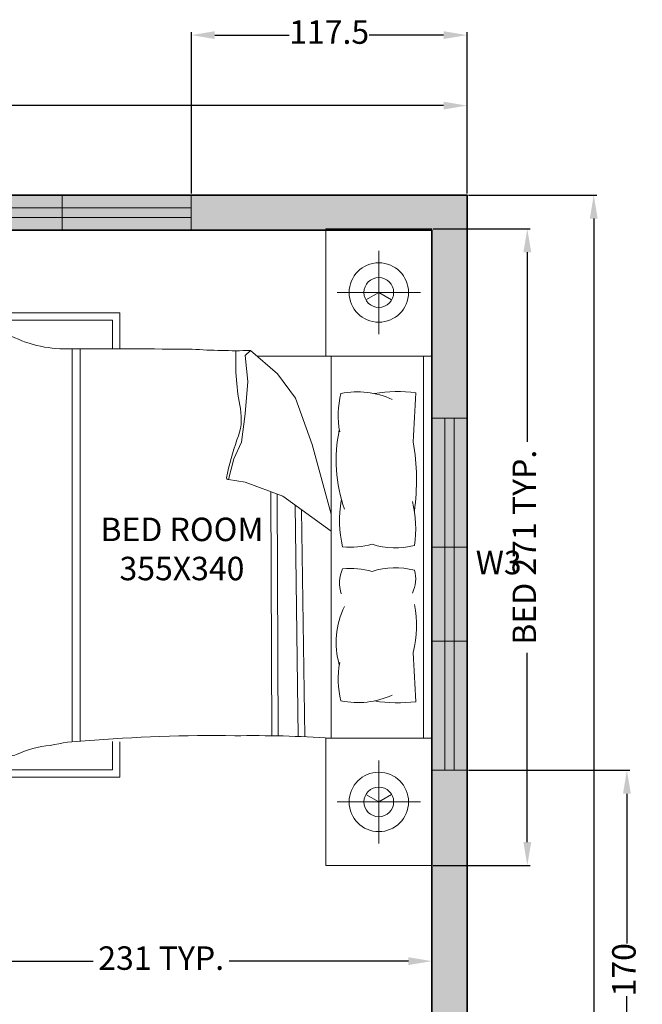
# Model space of a CAD drawing. Units: centimetres. Extents: x 2401 to 3632, y 2122 to 3526.
# Tile 10 of 10: x 3055 to 3320, y 3106 to 3526. Entities that reach past the tile are written whole.
import ezdxf

# ---------------------------------------------------------------- set-up
doc = ezdxf.new("R2010")
doc.units = ezdxf.units.CM
for name, color, linetype, lineweight in [('A-ANNO-DIMS', 9, 'Continuous', 18), ('A-ANNO-TEXT', 9, 'Continuous', 18), ('A-AREA-IDEN', 9, 'Continuous', 25), ('A-FURN', 9, 'Continuous', 18), ('A-GLAZ', 4, 'Continuous', 18), ('A-WALL', 7, 'Continuous', 35)]:
    doc.layers.add(name, color=color, linetype=linetype, lineweight=lineweight)
doc.layers.add('A-GLAZ-PATT', color=251, linetype='Continuous', lineweight=13, true_color=0x636466)
doc.layers.add('A-WALL-PATT', color=18, linetype='Continuous', lineweight=13, true_color=0x000000)
doc.styles.get("Standard").update_dxf_attribs({"font": 'arial.ttf'})
doc.dimstyles.new('ISO-25', dxfattribs={"dimtxt": 10, "dimasz": 10, "dimexe": 1.25, "dimexo": 0.625, "dimtad": 0, "dimtxsty": 'Standard', "dimcen": 2.5, "dimadec": 0, "dimazin": 0, "dimtfac": 1, "dimtmove": 0, "dimatfit": 3, "dimfxl": 1, "dimarcsym": 0})

# ---------------------------------------------------------------- blocks, each defined once
blk = doc.blocks.new('bed')
for p, q in [((3025.77, 3949.95), (3025.77, 3649.95)), ((3000.77, 3900.35), (3000.77, 3939.55)), ((2981.17, 3919.95), (3020.37, 3919.95)), ((2770.64, 3910.36), (2878.71, 3910.36)), ((2770.64, 3691.65), (2770.64, 3910.36)), ((2878.71, 3910.36), (2878.71, 3893.39)), ((2774.11, 3906.88), (2774.11, 3695.12)), ((2875.23, 3906.88), (2774.11, 3906.88)), ((2875.23, 3893.39), (2875.23, 3906.88)), ((2856.25, 3708.31), (2856.25, 3893.41)), ((2860, 3708.59), (2860, 3893.41)), ((2937.86, 3890.21), (2940.29, 3892.64)), ((2940.29, 3892.64), (2953.05, 3881.7)), ((2939.08, 3878.06), (2937.86, 3890.21)), ((3025.77, 3889.95), (2943.43, 3889.95)), ((2978.36, 3889.95), (2978.36, 3709.95)), ((3021.92, 3709.95), (3021.92, 3889.95)), ((2804.53, 3877.32), (2807.92, 3877.98)), ((2937.86, 3862.87), (2939.08, 3878.06)), ((2953.05, 3881.7), (2961.55, 3870.16)), ((2961.55, 3870.16), (2969.44, 3848.28)), ((2826.78, 3739.05), (2826.78, 3860.86)), ((2936.04, 3849.5), (2937.86, 3862.87)), ((2804.53, 3856.35), (2807.92, 3855.69)), ((2932.4, 3841.6), (2936.04, 3849.5)), ((2969.44, 3848.28), (2978.36, 3815.57)), ((2929.97, 3831.88), (2932.4, 3841.6)), ((2937.86, 3830.66), (2929.97, 3831.88)), ((2955.47, 3823.98), (2937.86, 3830.66)), ((2950.29, 3711.02), (2949.82, 3826.13)), ((2953.37, 3711.03), (2952.92, 3824.95)), ((2978.36, 3807.54), (2955.47, 3823.98)), ((2962.82, 3710.88), (2961.28, 3819.81)), ((2965.89, 3710.76), (2964.4, 3817.57)), ((2804.53, 3745.65), (2807.92, 3746.31)), ((2804.53, 3724.68), (2807.92, 3724.02)), ((2875.23, 3695.12), (2875.23, 3708.35)), ((2878.71, 3708.28), (2878.71, 3691.65)), ((3000.77, 3699.55), (3000.77, 3660.35)), ((2774.11, 3695.12), (2875.23, 3695.12)), ((2878.71, 3691.65), (2770.64, 3691.65)), ((2981.17, 3679.95), (3020.37, 3679.95))]:
    blk.add_line(p, q)
for points in [[(2975.77, 3889.95), (2975.77, 3949.95), (3025.77, 3949.95)], [(3000.77, 3919.95), (2994.7, 3916.45)], [(3000.77, 3919.95), (3006.83, 3916.45)], [(3025.77, 3709.95), (2975.77, 3709.95), (2975.77, 3649.95), (3025.77, 3649.95)], [(3000.77, 3679.95), (2994.7, 3683.45)], [(3000.77, 3679.95), (3006.83, 3683.45)]]:
    blk.add_lwpolyline(points)
for points in [[(2912.82, 3893.27, 0.001242), (2855.9, 3893.41, -0.127202), (2827.53, 3899.43)], [(3018.29, 3872.72, 0.074897), (2998.69, 3872.36, -0.472817)], [(2997.6, 3801.36, 0.14099), (3017.59, 3800.76, 0.235245)], [(2997.6, 3788.55, -0.14099), (3017.59, 3789.15, -0.235245)], [(3018.29, 3727.19, -0.074897), (2998.69, 3727.55, 0.472817)], [(2862.36, 3708.67, 0.056112), (2845.85, 3706.5, 0.095341), (2829.95, 3702.28)]]:
    blk.add_lwpolyline(points, format="xyb")
for centre, radius in [((3000.77, 3919.95), 14), ((3000.77, 3919.95), 7), ((2785.6, 3864.98), 0.764), ((2793.66, 3859.99), 0.764), ((2793.66, 3742.02), 0.764), ((2785.6, 3737.02), 0.764), ((3000.77, 3679.95), 14), ((3000.77, 3679.95), 7)]:
    blk.add_circle(centre, radius)
for centre, radius, start, end in [((2760.03, 3923.26), 23.79, 306.3036, 316.4814), ((2763.59, 3916.39), 19.09, 303.4617, 330.1116), ((2768.83, 3936.05), 39.18, 277.745, 311.8856), ((2764.96, 3869.02), 39.18, 34.3865, 68.5908), ((2827.73, 3896.66), 2.77, 93.98, 207.3412), ((2768, 3905.7), 15.93, 292.5547, 318.9546), ((2776.56, 3949.33), 54.2, 267.4081, 273.6519), ((2514.5, 3864.44), 312.3, 359.3433, 5.6887), ((2932.84, 4167.71), 275.17, 265.8294, 271.553), ((3046.53, 3887.51), 113.22, 177.4519, 191.3392), ((2796.37, 3886.9), 4.34, 77.7115, 159.0387), ((2794.02, 3891.25), 3.27, 238.4633, 358.2869), ((2804.75, 3884.63), 9.91, 138.8402, 177.9352), ((2798.78, 3888.31), 3.2, 117.6827, 223.7762), ((2798.06, 3887.99), 3.25, 2.9516, 103.728), ((2824.04, 3897.09), 27.41, 192.5173, 207.1824), ((2793.67, 3886.12), 6.19, 345.4653, 54.2343), ((2803, 3894.63), 6.69, 211.3827, 255.2969), ((2804.28, 3884.18), 4.5, 350.264, 160.8688), ((2799.41, 3885.11), 2.76, 333.9755, 53.2681), ((2815.84, 3882.53), 7.17, 84.9449, 172.8857), ((2816.56, 3884.61), 5.07, 354.4856, 91.0538), ((2805.66, 3897.83), 22.71, 303.6671, 333.2997), ((2795.33, 3884.97), 0.487, 177.9352, 11.4834), ((2795.58, 3885.02), 0.236, 11.4834, 127.9409), ((2796.77, 3886.39), 0.424, 223.7762, 159.7183), ((2805.64, 3885.26), 5.62, 175.969, 254.3045), ((2798.17, 3879.2), 5.99, 6.1662, 51.5825), ((2814.2, 3893.11), 14.16, 211.2614, 251.7045), ((2817.43, 3883.78), 8.71, 182.3591, 234.0401), ((2818.55, 3879.71), 6.96, 111.5819, 201.4221), ((2812.81, 3886.16), 9.02, 265.2933, 346.921), ((2813.05, 3893.24), 16.1, 236.2883, 266.5076), ((2810.99, 3881.04), 7.46, 209.9085, 343.1337), ((2824.57, 3889.51), 12.43, 238.8218, 279.1554), ((2819.17, 3867.4), 11.57, 55.785, 94.7304), ((2775.06, 3890.75), 28.48, 313.1541, 322.0459), ((2796.01, 3873.64), 0.586, 142.4737, 265.053), ((2796.78, 3873.76), 1.26, 127.7621, 169.0403), ((2796.11, 3874.82), 1.78, 265.053, 338.3618), ((2798.46, 3872.39), 2.32, 113.4276, 137.6104), ((2798.2, 3874.8), 0.764, 183.2768, 356.7232), ((2798.76, 3873.41), 1.25, 139.7889, 227.6792), ((2795.81, 3873.43), 2.5, 353.0852, 15.7171), ((2797.45, 3873.13), 1.58, 350.3487, 43.6538), ((2800.38, 3874.76), 1.84, 198.7263, 262.5032), ((2798.92, 3873.91), 0.73, 1.1081, 91.8675), ((2800.29, 3873.51), 0.59, 255.2356, 54.9248), ((2799.38, 3873.74), 1.27, 11.5637, 52.6358), ((2814.13, 3876.31), 1.86, 167.3041, 285.1471), ((2819.17, 3867.4), 11.57, 122.7011, 126.3445), ((2821.34, 3879.88), 9.56, 199.2822, 299.1751), ((2816.22, 3868.58), 6.15, 41.5653, 105.1471), ((2819.61, 3881.32), 8.62, 277.436, 299.9149), ((2823.47, 3874.11), 3.61, 30.0293, 52.325), ((2786.72, 3869.91), 0.853, 124.3538, 214.3923), ((2787.97, 3869.78), 1.99, 190.3057, 287.1958), ((2788.54, 3870.49), 2.31, 176.9701, 248.2913), ((2805.02, 3882.67), 22.32, 212.6784, 216.3746), ((2787.76, 3869.95), 0.883, 216.3746, 291.7548), ((2789.87, 3869.34), 1.99, 122.8155, 187.3992), ((2788.34, 3868.51), 0.666, 289.3605, 111.7548), ((2788.84, 3868.51), 0.666, 221.8703, 44.2646), ((2790.75, 3869.08), 2.31, 109.4799, 177.6828), ((2789.51, 3870.54), 0.853, 56.8636, 146.9021), ((2789.95, 3869.59), 0.883, 148.8844, 224.2646), ((2808.3, 3858.51), 22.32, 145.1882, 148.8844), ((2795.58, 3857.56), 12.46, 94.756, 119.2041), ((2822.1, 3839.62), 40.99, 132.2412, 142.1744), ((2801.41, 3872.25), 8.46, 178.3264, 187.1302), ((2792.27, 3871.07), 1.58, 11.3256, 64.4621), ((2797.62, 3873.34), 4.74, 190.2588, 210.656), ((2794.44, 3871.41), 1.44, 188.3432, 274.2869), ((2795.7, 3872.2), 2.51, 210.656, 242.6341), ((2797.6, 3874.36), 4.82, 218.2101, 226.3071), ((2794.04, 3870.31), 0.611, 325.7657, 67.4417), ((2796.2, 3845.18), 24.85, 73.5842, 93.8277), ((2798.36, 3872.98), 0.658, 227.6792, 350.3487), ((2811.5, 3870.46), 8.46, 178.3264, 187.1302), ((2802.37, 3869.29), 1.58, 11.3256, 64.4621), ((2807.71, 3871.55), 4.74, 190.2588, 210.656), ((2804.53, 3869.62), 1.44, 188.3432, 274.2869), ((2805.8, 3870.42), 2.51, 210.656, 242.6341), ((2807.7, 3872.58), 4.82, 218.2101, 226.3071), ((2804.13, 3868.53), 0.611, 325.7657, 67.4417), ((2824.18, 3875.64), 4.49, 221.5653, 293.8354), ((2823.47, 3874.11), 3.61, 314.4517, 333.558), ((3021.8, 3862.02), 40.2, 165.1039, 191.0369), ((2990.83, 3834.5), 38.67, 65.1316, 101.7583), ((5873.3, 3707.37), 2859.79, 176.68521, 177.14978), ((2783.42, 3863.83), 0.586, 142.4737, 265.053), ((2784.19, 3863.94), 1.26, 61.2196, 169.0403), ((2783.52, 3865.01), 1.78, 265.053, 338.3618), ((2785.02, 3866.54), 1.51, 157.4086, 261.4386), ((2784.17, 3866.59), 0.757, 58.0499, 135.6268), ((2785.87, 3862.58), 2.32, 113.4276, 137.6104), ((2784.96, 3866.11), 0.506, 172.906, 277.132), ((2783.3, 3865.19), 2.41, 14.7558, 58.0499), ((2786.17, 3863.6), 1.25, 139.7889, 227.6792), ((2786.67, 3865.83), 1.04, 36.1046, 181.4281), ((2783.22, 3863.62), 2.5, 353.0852, 15.7171), ((2784.86, 3863.32), 1.58, 350.3487, 43.6538), ((2787.79, 3864.95), 1.84, 198.7263, 262.5032), ((2786.06, 3866.65), 1.05, 270.0645, 331.1507), ((2786.96, 3866.4), 1.2, 221.8413, 265.7877), ((2786.33, 3864.09), 0.73, 1.1081, 91.8675), ((2786.95, 3865.94), 0.749, 263.7526, 41.7054), ((2786.79, 3863.93), 1.27, 11.5637, 86.365), ((2795.58, 3857.56), 12.46, 124.0033, 132.4917), ((2787.7, 3863.7), 0.59, 255.2356, 54.9248), ((2782.77, 3855.98), 13.31, 63.7819, 68.2913), ((2789.87, 3866.22), 2.12, 128.3208, 208.8162), ((2790.26, 3866.38), 2.53, 207.7043, 254.3516), ((2791.86, 3866.57), 3.48, 157.2305, 229.0635), ((2790.69, 3867.72), 2.05, 174.4544, 220.6188), ((2779.03, 3856.28), 14.94, 30.544, 49.818), ((2787.26, 3864.79), 2.46, 340.0041, 40.6188), ((2805.85, 3867.41), 1.44, 147.5332, 233.4768), ((2804.7, 3867.58), 0.611, 354.3784, 96.0543), ((2807.15, 3868.15), 2.51, 179.1859, 211.164), ((2796.2, 3845.18), 24.85, 63.0032, 69.8941), ((2809.06, 3869.3), 4.74, 211.164, 231.5612), ((2809.89, 3873.16), 8.46, 234.6898, 243.4936), ((2809.96, 3868.8), 4.82, 195.5129, 203.6099), ((2804.54, 3865.66), 1.58, 357.3579, 50.4944), ((2811.3, 3865.97), 0.578, 12.7051, 190.4384), ((2811.66, 3866.04), 0.94, 190.4384, 10.4136), ((2911.57, 3860.44), 24.42, 336.2616, 11.3392), ((2785.77, 3863.16), 0.658, 227.6792, 350.3487), ((2788.61, 3864.93), 3.48, 270.278, 342.111), ((2790.93, 3860.58), 2.46, 98.7227, 159.3375), ((2789.7, 3863.74), 2.53, 244.9899, 291.6373), ((2790.25, 3865.04), 2.05, 278.7227, 324.8872), ((2789.89, 3863.37), 2.12, 290.5253, 358.5375), ((2792.24, 3858.95), 1.26, 61.2196, 169.0403), ((2791.57, 3860.01), 1.78, 265.053, 338.3618), ((2793.07, 3861.54), 1.51, 157.4086, 261.4386), ((2792.22, 3861.59), 0.757, 58.0499, 135.6268), ((2794.02, 3863.97), 2.12, 182.8499, 266.1226), ((2793.19, 3865.47), 2.05, 231.7607, 277.9252), ((2794.79, 3865.83), 3.48, 214.5369, 286.3699), ((2793.92, 3857.58), 2.32, 113.4276, 137.6104), ((2793.01, 3861.12), 0.506, 172.906, 277.132), ((2791.35, 3860.19), 2.41, 14.7558, 58.0499), ((2779.03, 3856.28), 14.94, 23.0501, 23.8477), ((2794.22, 3858.6), 1.25, 139.7889, 227.6792), ((2793.81, 3861), 2.46, 37.3105, 97.9252), ((2794.72, 3860.83), 1.04, 36.1046, 181.4281), ((2791.27, 3858.62), 2.5, 353.0852, 15.7171), ((2794.09, 3864.38), 2.53, 265.0106, 311.658), ((2792.91, 3858.32), 1.58, 350.3487, 43.6538), ((2795.84, 3859.95), 1.84, 198.7263, 262.5032), ((2794.11, 3861.65), 1.05, 270.0645, 331.1507), ((2795.01, 3861.4), 1.2, 221.8413, 265.7877), ((2794.38, 3859.1), 0.73, 1.1081, 91.8675), ((2795, 3860.95), 0.749, 263.7526, 41.7054), ((2794.84, 3858.93), 1.27, 11.5637, 86.365), ((2810.99, 3852.63), 7.46, 16.8663, 150.0915), ((2821.34, 3853.79), 9.56, 60.8249, 160.7178), ((2816.22, 3865.09), 6.15, 254.8529, 318.4347), ((2819.61, 3852.35), 8.62, 60.0851, 82.564), ((2824.18, 3858.03), 4.49, 66.1646, 138.4347), ((2823.47, 3859.56), 3.61, 23.229, 45.5483), ((2791.47, 3858.83), 0.586, 142.4737, 265.053), ((2793.82, 3858.17), 0.658, 227.6792, 350.3487), ((2779.03, 3856.28), 14.94, 357.1071, 4.7585), ((2795.75, 3858.7), 0.59, 255.2356, 54.9248), ((2813.05, 3840.43), 16.1, 93.4924, 123.7117), ((2817.43, 3849.89), 8.71, 125.9599, 177.6409), ((2818.55, 3853.96), 6.96, 158.5779, 248.4181), ((2812.81, 3847.51), 9.02, 13.079, 94.7067), ((2814.13, 3857.35), 1.86, 74.8529, 192.6959), ((2819.17, 3866.26), 11.57, 233.6555, 237.2989), ((2824.57, 3844.16), 12.43, 79.7133, 121.1782), ((2819.17, 3866.26), 11.57, 265.2696, 304.215), ((2805.66, 3835.83), 22.71, 21.4941, 56.3329), ((2823.47, 3859.56), 3.61, 307.675, 336.7144), ((3050.38, 3840.86), 69.73, 168.0397, 199.2615), ((2805.64, 3848.41), 5.62, 105.6955, 184.031), ((2804.28, 3849.49), 4.5, 199.1312, 9.736), ((2798.17, 3854.46), 5.99, 308.4175, 353.8338), ((2814.2, 3840.56), 14.16, 108.2955, 148.7386), ((2815.84, 3851.14), 7.17, 187.1143, 275.0551), ((3043.34, 3811.05), 116.34, 160.1194, 169.3383), ((2794.02, 3842.42), 3.27, 1.7131, 121.5367), ((2795.33, 3848.7), 0.487, 348.5166, 182.0648), ((2804.75, 3849.04), 9.91, 182.0648, 221.1598), ((2795.58, 3848.65), 0.236, 232.0591, 348.5166), ((2798.78, 3845.36), 3.2, 136.2238, 242.3173), ((2796.93, 3847.24), 0.255, 200.2667, 136.2271), ((2793.67, 3847.55), 6.19, 305.7657, 14.5347), ((2824.04, 3836.58), 27.41, 152.8176, 167.4827), ((2798.06, 3845.68), 3.25, 256.272, 357.0484), ((2803, 3839.04), 6.69, 104.7031, 148.6173), ((2799.41, 3848.56), 2.76, 306.7319, 26.0245), ((2816.56, 3849.06), 5.07, 268.9462, 5.5144), ((2909.73, 3831.62), 108.8, 352.2196, 9.497), ((2768, 3827.97), 15.93, 41.0454, 67.4453), ((2764.96, 3864.65), 39.18, 291.4092, 325.6135), ((2796.37, 3846.77), 4.34, 200.9613, 282.2885), ((2776.56, 3784.33), 54.2, 86.3481, 92.5919), ((2768.83, 3797.62), 39.18, 4.4623, 82.255), ((2763.59, 3817.28), 19.09, 1.272, 56.5383), ((2929.73, 3832.56), 0.724, 178.8623, 289.7536), ((2760.03, 3810.41), 23.79, 17.8504, 53.6964), ((2753.34, 3797.91), 35.39, 34.0123, 54.053), ((2753.52, 3811.58), 21.54, 343.5431, 17.0202), ((2747.85, 3800.62), 39.18, 4.4623, 27.4146), ((3035.15, 3812.63), 52.9, 169.8617, 193.6238), ((2964.72, 3808.64), 53.46, 351.5249, 13.96), ((2742.41, 3803.04), 31.85, 4.3787, 5.6357), ((2720.59, 3786.27), 56.92, 19.7217, 19.9028), ((2783.99, 3800.45), 4.34, 47.7873, 129.1145), ((2784.12, 3805.39), 3.27, 208.5391, 328.3627), ((2790.12, 3794.3), 9.91, 108.9159, 148.011), ((2786.78, 3800.47), 3.2, 87.7585, 193.852), ((2813.06, 3795.47), 27.41, 162.593, 177.2582), ((2781.26, 3801.12), 6.19, 315.5411, 24.3101), ((2793.6, 3803.84), 6.69, 181.4585, 225.3727), ((2786, 3800.55), 3.25, 333.0274, 73.8037), ((2782.13, 3799.29), 0.487, 148.011, 341.5592), ((2782.37, 3799.21), 0.236, 341.5592, 98.0167), ((2784.08, 3799.8), 0.424, 193.852, 129.9245), ((2804.97, 3797.45), 4.34, 47.7873, 129.1145), ((2805.11, 3802.39), 3.27, 208.5391, 328.3627), ((2811.1, 3791.3), 9.91, 108.9159, 148.011), ((2807.77, 3797.47), 3.2, 87.7585, 193.852), ((2802.25, 3798.12), 6.19, 315.5411, 24.3101), ((2834.04, 3792.47), 27.41, 162.593, 177.2582), ((2806.98, 3797.55), 3.25, 333.0274, 73.8037), ((2814.58, 3800.84), 6.69, 181.4585, 225.3727), ((2987.57, 3836.72), 36.76, 264.0129, 285.8293), ((2813.06, 3796.53), 27.41, 182.7418, 197.407), ((2781.26, 3790.88), 6.19, 335.6899, 44.4589), ((2803.11, 3796.29), 0.487, 148.011, 341.5592), ((2803.11, 3795.71), 0.487, 18.4408, 211.989), ((2811.1, 3800.7), 9.91, 211.989, 251.0841), ((2803.35, 3796.21), 0.236, 341.5592, 98.0167), ((2803.35, 3795.79), 0.236, 261.9833, 18.4408), ((2807.77, 3794.53), 3.2, 166.148, 272.2415), ((2805.07, 3796.8), 0.424, 193.852, 129.9245), ((2805.23, 3795.24), 0.255, 230.1909, 166.0209), ((2802.25, 3793.88), 6.19, 335.6899, 44.4589), ((2834.04, 3799.53), 27.41, 182.7418, 197.407), ((2806.98, 3794.45), 3.25, 286.1963, 26.9726), ((2814.58, 3791.16), 6.69, 134.6273, 178.5415), ((2777.88, 3795.65), 30.32, 262.8636, 351.8197), ((2784.12, 3786.62), 3.27, 31.6373, 151.4609), ((2782.13, 3792.71), 0.487, 18.4408, 211.989), ((2790.12, 3797.71), 9.91, 211.989, 251.0841), ((2782.37, 3792.79), 0.236, 261.9833, 18.4408), ((2786.78, 3791.54), 3.2, 166.148, 272.2415), ((2784.25, 3792.24), 0.255, 230.1909, 166.0209), ((2793.6, 3788.16), 6.69, 134.6273, 178.5415), ((2786, 3791.45), 3.25, 286.1963, 26.9726), ((2805.11, 3789.62), 3.27, 31.6373, 151.4609), ((2804.97, 3794.55), 4.34, 230.8855, 312.2127), ((2998.15, 3783.03), 15.9, 155.0183, 198.5407), ((2987.57, 3753.18), 36.76, 74.1707, 95.9871), ((2753.52, 3780.42), 21.54, 342.9798, 16.4569), ((2742.41, 3788.96), 31.85, 354.3643, 355.6213), ((2720.59, 3805.74), 56.92, 340.0972, 340.2783), ((2783.99, 3791.55), 4.34, 230.8855, 312.2127), ((2747.85, 3791.38), 39.18, 332.5854, 355.5377), ((3003.33, 3785.03), 14.84, 333.3437, 16.1026), ((2780.65, 3791.73), 17.54, 248.117, 276.6195), ((2775.77, 3775.64), 7.03, 256.3898, 349.0739), ((2776.73, 3780.92), 8.89, 252.8609, 311.9049), ((2764.96, 3737.36), 39.18, 34.3865, 68.5908), ((3018.84, 3755.24), 38.19, 153.8761, 196.1746), ((2965.8, 3762.79), 52.74, 346.3427, 11.1841), ((2776.56, 3817.67), 54.2, 267.4081, 273.6519), ((2768, 3774.04), 15.93, 292.5547, 318.9546), ((2796.37, 3755.24), 4.34, 77.7115, 159.0387), ((2794.02, 3759.58), 3.27, 238.4633, 358.2869), ((2804.75, 3752.96), 9.91, 138.8402, 177.9352), ((2798.78, 3756.64), 3.2, 117.6827, 223.7762), ((2798.06, 3756.33), 3.25, 2.9516, 103.728), ((2803, 3762.97), 6.69, 211.3827, 255.2969), ((2793.67, 3754.46), 6.19, 345.4653, 54.2343), ((2824.04, 3765.42), 27.41, 192.5173, 207.1824), ((2815.84, 3750.86), 7.17, 84.9449, 172.8857), ((2816.56, 3752.94), 5.07, 354.4856, 91.0538), ((2805.66, 3766.17), 22.71, 303.6671, 338.5059), ((2795.33, 3753.3), 0.487, 177.9352, 11.4834), ((2795.58, 3753.35), 0.236, 11.4834, 127.9409), ((2796.77, 3754.72), 0.424, 223.7762, 159.7183), ((2805.64, 3753.59), 5.62, 175.969, 254.3045), ((2804.28, 3752.51), 4.5, 350.264, 160.8688), ((2799.41, 3753.44), 2.76, 333.9755, 53.2681), ((2814.2, 3761.44), 14.16, 211.2614, 251.7045), ((2818.55, 3748.05), 6.96, 111.5819, 201.4221), ((2798.17, 3747.54), 5.99, 6.1662, 51.5825), ((2813.05, 3761.57), 16.1, 236.2883, 266.5076), ((2817.43, 3752.11), 8.71, 182.3591, 234.0401), ((2812.81, 3754.5), 9.02, 265.2933, 346.921), ((5873.3, 3892.54), 2859.79, 182.85022, 183.31479), ((2791.47, 3743.17), 0.586, 94.947, 217.5263), ((2791.57, 3741.99), 1.78, 21.6382, 94.947), ((2794.22, 3743.4), 1.25, 132.3208, 220.2111), ((2793.82, 3743.84), 0.658, 9.6513, 132.3208), ((2791.27, 3743.38), 2.5, 344.2829, 6.9148), ((2779.03, 3745.73), 14.94, 355.2415, 2.8929), ((2792.91, 3743.68), 1.58, 316.3462, 9.6513), ((2795.84, 3742.05), 1.84, 97.4968, 161.2737), ((2795.75, 3743.3), 0.59, 305.0752, 104.7644), ((2810.99, 3749.37), 7.46, 209.9085, 343.1337), ((2814.13, 3744.65), 1.86, 167.3041, 285.1471), ((2819.17, 3735.74), 11.57, 122.7011, 126.3445), ((2821.34, 3748.21), 9.56, 199.2822, 299.1751), ((2824.57, 3757.84), 12.43, 238.8218, 280.2867), ((2819.17, 3735.74), 11.57, 55.785, 94.7304), ((2823.47, 3742.45), 3.61, 23.2856, 52.325), ((3021.8, 3737.89), 40.2, 168.9631, 194.8961), ((2783.42, 3738.18), 0.586, 94.947, 217.5263), ((2783.52, 3736.99), 1.78, 21.6382, 94.947), ((2786.17, 3738.4), 1.25, 132.3208, 220.2111), ((2785.77, 3738.84), 0.658, 9.6513, 132.3208), ((2783.22, 3738.38), 2.5, 344.2829, 6.9148), ((2784.86, 3738.68), 1.58, 316.3462, 9.6513), ((2787.79, 3737.05), 1.84, 97.4968, 161.2737), ((2787.7, 3738.3), 0.59, 305.0752, 104.7644), ((2789.7, 3738.26), 2.53, 68.3627, 115.0101), ((2788.61, 3737.07), 3.48, 17.889, 89.722), ((2790.93, 3741.42), 2.46, 200.6625, 261.2773), ((2790.25, 3736.96), 2.05, 35.1128, 81.2773), ((2789.89, 3738.63), 2.12, 1.4625, 69.4747), ((2792.24, 3743.06), 1.26, 190.9597, 298.7804), ((2793.07, 3740.46), 1.51, 98.5614, 202.5914), ((2792.22, 3740.41), 0.757, 224.3732, 301.9501), ((2794.02, 3738.03), 2.12, 93.8774, 177.1501), ((2794.79, 3736.17), 3.48, 73.6301, 145.4631), ((2793.92, 3744.42), 2.32, 222.3896, 246.5724), ((2793.01, 3740.89), 0.506, 82.868, 187.094), ((2791.35, 3741.81), 2.41, 301.9501, 345.2442), ((2779.03, 3745.73), 14.94, 336.1523, 336.9499), ((2793.81, 3741), 2.46, 262.0748, 322.6895), ((2794.72, 3741.17), 1.04, 178.5719, 323.8954), ((2794.09, 3737.62), 2.53, 48.342, 94.9894), ((2795.01, 3740.6), 1.2, 94.2123, 138.1587), ((2794.11, 3740.35), 1.05, 28.8493, 89.9355), ((2794.38, 3742.91), 0.73, 268.1325, 358.8919), ((2794.84, 3743.07), 1.27, 273.635, 348.4363), ((2795, 3741.06), 0.749, 318.2946, 96.2474), ((2816.22, 3736.91), 6.15, 41.5653, 105.1471), ((2819.61, 3749.66), 8.62, 277.436, 299.9149), ((2824.18, 3743.97), 4.49, 221.5653, 293.8354), ((2535.01, 3729.86), 291.92, 355.2402, 1.8035), ((2823.47, 3742.45), 3.61, 314.4517, 336.7144), ((2784.19, 3738.06), 1.26, 190.9597, 298.7804), ((2785.02, 3735.46), 1.51, 98.5614, 202.5914), ((2784.17, 3735.41), 0.757, 224.3732, 301.9501), ((2785.87, 3739.42), 2.32, 222.3896, 246.5724), ((2784.96, 3735.89), 0.506, 82.868, 187.094), ((2783.3, 3736.82), 2.41, 301.9501, 345.2442), ((2786.67, 3736.18), 1.04, 178.5719, 323.8954), ((2787.97, 3732.22), 1.99, 72.8042, 169.6943), ((2786.96, 3735.61), 1.2, 94.2123, 138.1587), ((2786.06, 3735.36), 1.05, 28.8493, 89.9355), ((2786.33, 3737.91), 0.73, 268.1325, 358.8919), ((2786.79, 3738.08), 1.27, 273.635, 348.4363), ((2786.95, 3736.06), 0.749, 318.2946, 96.2474), ((2795.58, 3744.44), 12.46, 227.5083, 235.9967), ((2782.77, 3746.02), 13.31, 291.7087, 296.2181), ((2789.87, 3735.78), 2.12, 151.1838, 231.6792), ((2790.26, 3735.62), 2.53, 105.6484, 152.2957), ((2788.34, 3733.49), 0.666, 248.2452, 70.6395), ((2788.84, 3733.49), 0.666, 315.7354, 138.1297), ((2791.86, 3735.43), 3.48, 130.9365, 202.7695), ((2790.69, 3734.28), 2.05, 139.3812, 185.5456), ((2779.03, 3745.73), 14.94, 310.182, 329.456), ((2787.26, 3737.22), 2.46, 319.3812, 19.9959), ((2822.1, 3762.38), 40.99, 217.8256, 227.7588), ((2793.19, 3736.53), 2.05, 82.0748, 128.2393), ((2805.85, 3734.59), 1.44, 126.5232, 212.4668), ((2807.15, 3733.85), 2.51, 148.836, 180.8141), ((2804.7, 3734.43), 0.611, 263.9457, 5.6216), ((2796.2, 3756.82), 24.85, 290.1059, 296.9968), ((2809.06, 3732.7), 4.74, 128.4388, 148.836), ((2809.89, 3728.84), 8.46, 116.5064, 125.3102), ((2809.96, 3733.2), 4.82, 156.3901, 164.4871), ((2804.54, 3736.34), 1.58, 309.5056, 2.6421), ((2811.3, 3736.03), 0.578, 169.5616, 347.2949), ((2811.66, 3735.96), 0.94, 349.5864, 169.5616), ((2786.72, 3732.09), 0.853, 145.6077, 235.6462), ((2788.54, 3731.51), 2.31, 111.7087, 183.0299), ((2805.02, 3719.34), 22.32, 143.6254, 147.3216), ((2787.76, 3732.05), 0.883, 68.2452, 143.6254), ((2789.87, 3732.67), 1.99, 172.6008, 237.1845), ((2790.75, 3732.92), 2.31, 182.3172, 250.5201), ((2789.51, 3731.46), 0.853, 213.0979, 303.1364), ((2789.95, 3732.41), 0.883, 135.7354, 211.1156), ((2808.3, 3743.49), 22.32, 211.1156, 214.8118), ((2795.58, 3744.44), 12.46, 240.7959, 265.244), ((2797.62, 3728.66), 4.74, 149.344, 169.7412), ((2801.41, 3729.75), 8.46, 172.8698, 181.6736), ((2792.27, 3730.93), 1.58, 295.5379, 348.6744), ((2794.44, 3730.6), 1.44, 85.7131, 171.6568), ((2795.7, 3729.8), 2.51, 117.3659, 149.344), ((2797.6, 3727.64), 4.82, 133.6929, 141.7899), ((2794.04, 3731.69), 0.611, 292.5583, 34.2343), ((2796.2, 3756.82), 24.85, 266.1723, 286.4158), ((2775.06, 3711.25), 28.48, 37.9541, 46.8459), ((2798.76, 3728.59), 1.25, 132.3208, 220.2111), ((2798.36, 3729.03), 0.658, 9.6513, 132.3208), ((2811.5, 3731.54), 8.46, 172.8698, 181.6736), ((2807.71, 3730.45), 4.74, 149.344, 169.7412), ((2802.37, 3732.72), 1.58, 295.5379, 348.6744), ((2804.53, 3732.38), 1.44, 85.7131, 171.6568), ((2805.8, 3731.59), 2.51, 117.3659, 149.344), ((2807.7, 3729.43), 4.82, 133.6929, 141.7899), ((2804.13, 3733.47), 0.611, 292.5583, 34.2343), ((2821.34, 3722.12), 9.56, 60.8249, 160.7178), ((2824.18, 3726.36), 4.49, 66.1646, 138.4347), ((2823.47, 3727.89), 3.61, 16.6343, 45.5483), ((2990.83, 3765.41), 38.67, 258.2417, 294.8684), ((2796.01, 3728.36), 0.586, 94.947, 217.5263), ((2796.78, 3728.25), 1.26, 190.9597, 232.2379), ((2796.11, 3727.18), 1.78, 21.6382, 94.947), ((2798.46, 3729.61), 2.32, 222.3896, 246.5724), ((2798.2, 3727.21), 0.764, 3.2768, 176.7232), ((2795.81, 3728.57), 2.5, 344.2829, 6.9148), ((2797.45, 3728.87), 1.58, 316.3462, 9.6513), ((2800.38, 3727.24), 1.84, 97.4968, 161.2737), ((2798.92, 3728.1), 0.73, 268.1325, 358.8919), ((2800.29, 3728.49), 0.59, 305.0752, 104.7644), ((2799.38, 3728.26), 1.27, 307.3642, 348.4363), ((2813.05, 3708.76), 16.1, 93.4924, 123.7117), ((2810.99, 3720.97), 7.46, 16.8663, 150.0915), ((2817.43, 3718.23), 8.71, 125.9599, 177.6409), ((2818.55, 3722.29), 6.96, 158.5779, 248.4181), ((2812.81, 3715.84), 9.02, 13.079, 94.7067), ((2814.13, 3725.69), 1.86, 74.8529, 192.6959), ((2819.17, 3734.6), 11.57, 233.6555, 237.2989), ((2816.22, 3733.42), 6.15, 254.8529, 318.4347), ((2824.57, 3712.5), 12.43, 79.249, 121.1782), ((2819.17, 3734.6), 11.57, 265.2696, 304.215), ((2819.61, 3720.68), 8.62, 60.0851, 82.564), ((2823.47, 3727.89), 3.61, 307.675, 342.5814), ((2805.64, 3716.74), 5.62, 105.6955, 184.031), ((2798.17, 3722.8), 5.99, 308.4175, 353.8338), ((2814.2, 3708.9), 14.16, 108.2955, 148.7386), ((2805.66, 3704.17), 22.71, 23.6453, 56.3329), ((2795.33, 3717.04), 0.487, 348.5166, 182.0648), ((2804.75, 3717.37), 9.91, 182.0648, 221.1598), ((2795.58, 3716.99), 0.236, 232.0591, 348.5166), ((2798.78, 3713.69), 3.2, 136.2238, 242.3173), ((2796.93, 3715.57), 0.255, 200.2667, 136.2271), ((2824.04, 3704.91), 27.41, 152.8176, 167.4827), ((2793.67, 3715.88), 6.19, 305.7657, 14.5347), ((2804.28, 3717.82), 4.5, 199.1312, 9.736), ((2799.41, 3716.9), 2.76, 306.7319, 26.0245), ((2815.84, 3719.47), 7.17, 187.1143, 275.0551), ((2816.56, 3717.4), 5.07, 268.9462, 5.5144), ((2768, 3696.3), 15.93, 41.0454, 67.4453), ((2764.96, 3732.98), 39.18, 291.4092, 325.6135), ((2794.02, 3710.76), 3.27, 1.7131, 121.5367), ((2796.37, 3715.1), 4.34, 200.9613, 282.2885), ((2803, 3707.37), 6.69, 104.7031, 148.6173), ((2798.06, 3714.01), 3.25, 256.272, 357.0484), ((2922.1, 3008.05), 703.17, 89.11454, 94.87351), ((2941.69, 3172.15), 539.05, 86.1, 90.9282), ((2776.56, 3652.67), 54.2, 86.3481, 92.5919), ((2768.83, 3665.96), 39.18, 48.1144, 82.255), ((2828.43, 3704.55), 2.73, 156.5219, 303.8264), ((2763.59, 3685.61), 19.09, 29.8884, 56.5383), ((2760.03, 3678.74), 23.79, 43.5186, 53.6964)]:
    blk.add_arc(centre, radius, start, end)
blk = doc.blocks.new('*D14')
at = {"layer": 'A-ANNO-DIMS', "color": 0, "lineweight": -2, "transparency": 16777216}
for p, q in [((3246.06, 3451.1), (3300.7, 3451.1)), ((3299.45, 3441.1), (3299.45, 2946.17)), ((3299.45, 2421.1), (3299.45, 2916.04)), ((3246.06, 2411.1), (3300.7, 2411.1))]:
    blk.add_line(p, q, dxfattribs=at)
at = {"layer": 'A-ANNO-DIMS', "color": 0, "transparency": 16777216}
for points in [[(3297.79, 3441.1), (3301.12, 3441.1), (3299.45, 3451.1)], [(3297.79, 2421.1), (3301.12, 2421.1), (3299.45, 2411.1)]]:
    blk.add_solid(points, dxfattribs=at)
at = {"layer": 'Defpoints', "color": 0, "transparency": 16777216}
for p in [(3245.44, 3451.1), (3245.44, 2411.1), (3299.45, 2411.1)]:
    blk.add_point(p, dxfattribs=at)
at = {"layer": 'A-ANNO-DIMS', "color": 0, "transparency": 16777216, "insert": (3299.45, 2931.1), "char_height": 10, "attachment_point": 5, "rotation": 90}
blk.add_mtext('1040', dxfattribs=at)
blk = doc.blocks.new('*D17')
at = {"layer": 'A-ANNO-DIMS', "color": 0, "lineweight": -2, "transparency": 16777216}
for p, q in [((2500.44, 3451.73), (2500.44, 3490.46)), ((3245.44, 3451.73), (3245.44, 3490.46)), ((2510.44, 3489.21), (2861.27, 3489.21)), ((3235.44, 3489.21), (2884.6, 3489.21))]:
    blk.add_line(p, q, dxfattribs=at)
at = {"layer": 'A-ANNO-DIMS', "color": 0, "transparency": 16777216}
for points in [[(2510.44, 3490.88), (2510.44, 3487.55), (2500.44, 3489.21)], [(3235.44, 3490.88), (3235.44, 3487.55), (3245.44, 3489.21)]]:
    blk.add_solid(points, dxfattribs=at)
at = {"layer": 'Defpoints', "color": 0, "transparency": 16777216}
for p in [(3245.44, 3489.21), (2500.44, 3451.1), (3245.44, 3451.1)]:
    blk.add_point(p, dxfattribs=at)
at = {"layer": 'A-ANNO-DIMS', "color": 0, "transparency": 16777216, "insert": (2872.94, 3489.21), "char_height": 10, "attachment_point": 5}
blk.add_mtext('745', dxfattribs=at)
blk = doc.blocks.new('WIN-1500-3P')
for p, q in [((0, 15), (0, 0)), ((55, 15), (55, 0)), ((95, 15), (95, 0)), ((150, 15), (150, 0)), ((0, 9.5), (150, 9.5)), ((0, 5.5), (150, 5.5))]:
    blk.add_line(p, q)
blk = doc.blocks.new('*D24')
at = {"layer": 'A-ANNO-DIMS', "color": 0, "lineweight": -2, "transparency": 16777216}
for p, q in [((3231.06, 3436.73), (3272.38, 3436.73)), ((3271.13, 3426.73), (3271.13, 3346.03)), ((3271.13, 3175.47), (3271.13, 3256.17)), ((3231.06, 3165.47), (3272.38, 3165.47))]:
    blk.add_line(p, q, dxfattribs=at)
at = {"layer": 'A-ANNO-DIMS', "color": 0, "transparency": 16777216}
for points in [[(3269.46, 3426.73), (3272.79, 3426.73), (3271.13, 3436.73)], [(3269.46, 3175.47), (3272.79, 3175.47), (3271.13, 3165.47)]]:
    blk.add_solid(points, dxfattribs=at)
at = {"layer": 'Defpoints', "color": 0, "transparency": 16777216}
for p in [(3230.44, 3436.73), (3271.13, 3436.73), (3230.44, 3165.47)]:
    blk.add_point(p, dxfattribs=at)
at = {"layer": 'A-ANNO-DIMS', "color": 0, "transparency": 16777216, "insert": (3271.13, 3301.1), "char_height": 10, "attachment_point": 5, "rotation": 90}
blk.add_mtext('BED 271 TYP.', dxfattribs=at)
blk = doc.blocks.new('*D25')
at = {"layer": 'A-ANNO-DIMS', "color": 0, "lineweight": -2, "transparency": 16777216}
for p, q in [((2999.75, 3164.85), (2999.75, 3123.53)), ((3230.44, 3164.85), (3230.44, 3123.53)), ((3009.75, 3124.78), (3086.16, 3124.78)), ((3220.44, 3124.78), (3144.02, 3124.78))]:
    blk.add_line(p, q, dxfattribs=at)
at = {"layer": 'A-ANNO-DIMS', "color": 0, "transparency": 16777216}
for points in [[(3009.75, 3126.45), (3009.75, 3123.12), (2999.75, 3124.78)], [(3220.44, 3126.45), (3220.44, 3123.12), (3230.44, 3124.78)]]:
    blk.add_solid(points, dxfattribs=at)
at = {"layer": 'Defpoints', "color": 0, "transparency": 16777216}
for p in [(2999.75, 3165.47), (3230.44, 3165.47), (3230.44, 3124.78)]:
    blk.add_point(p, dxfattribs=at)
at = {"layer": 'A-ANNO-DIMS', "color": 0, "transparency": 16777216, "insert": (3115.09, 3124.78), "char_height": 10, "attachment_point": 5}
blk.add_mtext('231 TYP.', dxfattribs=at)
blk = doc.blocks.new('*D45')
at = {"layer": 'A-ANNO-DIMS', "color": 0, "lineweight": -2, "transparency": 16777216}
for p, q in [((3246.06, 3206.1), (3314.84, 3206.1)), ((3313.59, 3196.1), (3313.59, 3132.29)), ((3313.59, 3046.1), (3313.59, 3109.92)), ((3246.06, 3036.1), (3314.84, 3036.1))]:
    blk.add_line(p, q, dxfattribs=at)
at = {"layer": 'A-ANNO-DIMS', "color": 0, "transparency": 16777216}
for points in [[(3311.92, 3196.1), (3315.25, 3196.1), (3313.59, 3206.1)], [(3311.92, 3046.1), (3315.25, 3046.1), (3313.59, 3036.1)]]:
    blk.add_solid(points, dxfattribs=at)
at = {"layer": 'Defpoints', "color": 0, "transparency": 16777216}
for p in [(3245.44, 3206.1), (3313.59, 3206.1), (3245.44, 3036.1)]:
    blk.add_point(p, dxfattribs=at)
at = {"layer": 'A-ANNO-DIMS', "color": 0, "transparency": 16777216, "insert": (3313.59, 3121.1), "char_height": 10, "attachment_point": 5, "rotation": 90}
blk.add_mtext('170', dxfattribs=at)
blk = doc.blocks.new('*D46')
at = {"layer": 'A-ANNO-DIMS', "color": 0, "lineweight": -2, "transparency": 16777216}
for p, q in [((3127.94, 3451.73), (3127.94, 3520.5)), ((3137.94, 3519.25), (3169.62, 3519.25)), ((3235.44, 3519.25), (3203.75, 3519.25)), ((3245.44, 3451.73), (3245.44, 3520.5))]:
    blk.add_line(p, q, dxfattribs=at)
at = {"layer": 'A-ANNO-DIMS', "color": 0, "transparency": 16777216}
for points in [[(3137.94, 3520.92), (3137.94, 3517.59), (3127.94, 3519.25)], [(3235.44, 3520.92), (3235.44, 3517.59), (3245.44, 3519.25)]]:
    blk.add_solid(points, dxfattribs=at)
at = {"layer": 'Defpoints', "color": 0, "transparency": 16777216}
for p in [(3245.44, 3519.25), (3127.94, 3451.1), (3245.44, 3451.1)]:
    blk.add_point(p, dxfattribs=at)
at = {"layer": 'A-ANNO-DIMS', "color": 0, "transparency": 16777216, "insert": (3186.69, 3519.25), "char_height": 10, "attachment_point": 5}
blk.add_mtext('117.5', dxfattribs=at)

msp = doc.modelspace()

# ---------------------------------------------------------------- hatches: boundary and pattern name
at = {"layer": 'A-GLAZ-PATT'}
h = msp.add_hatch(color=256, dxfattribs=at)
h.dxf.hatch_style = 1
h.paths.add_polyline_path([(2505.936, 3356.104), (2500.436, 3356.104), (2500.436, 3301.104), (2505.936, 3301.104)])
h.paths.add_polyline_path([(2509.936, 3356.104), (2505.936, 3356.104), (2505.936, 3301.104), (2509.936, 3301.104)])
h.paths.add_polyline_path([(2515.436, 3335.674), (2515.436, 3356.104), (2509.936, 3356.104), (2509.936, 3301.104), (2515.436, 3301.104)])
h.paths.add_polyline_path([(2509.936, 3301.104), (2505.936, 3301.104), (2505.936, 3261.104), (2509.936, 3261.104)])
h.paths.add_polyline_path([(2515.436, 3301.104), (2509.936, 3301.104), (2509.936, 3261.104), (2515.436, 3261.104)])
h.paths.add_polyline_path([(2505.936, 3301.104), (2500.436, 3301.104), (2500.436, 3261.104), (2505.936, 3261.104)])
h.paths.add_polyline_path([(2515.436, 3261.104), (2509.936, 3261.104), (2509.936, 3206.104), (2515.436, 3206.104)])
h.paths.add_polyline_path([(2505.936, 3261.104), (2500.436, 3261.104), (2500.436, 3206.104), (2505.936, 3206.104)])
h.paths.add_polyline_path([(2509.936, 3261.104), (2505.936, 3261.104), (2505.936, 3206.104), (2509.936, 3206.104)])
h.paths.add_polyline_path([(3127.936, 3451.104), (3072.936, 3451.104), (3072.936, 3445.604), (3127.936, 3445.604)])
h.paths.add_polyline_path([(3032.936, 3441.604), (2977.936, 3441.604), (2977.936, 3436.104), (3032.936, 3436.104)])
h.paths.add_polyline_path([(3032.936, 3451.104), (2977.936, 3451.104), (2977.936, 3445.604), (3032.936, 3445.604)])
h.paths.add_polyline_path([(3032.936, 3445.604), (2977.936, 3445.604), (2977.936, 3441.604), (3032.936, 3441.604)])
h.paths.add_polyline_path([(3072.936, 3451.104), (3032.936, 3451.104), (3032.936, 3445.604), (3072.936, 3445.604)])
h.paths.add_polyline_path([(3072.936, 3445.604), (3032.936, 3445.604), (3032.936, 3441.604), (3072.936, 3441.604)])
h.paths.add_polyline_path([(3072.936, 3441.604), (3032.936, 3441.604), (3032.936, 3436.104), (3072.936, 3436.104)])
h.paths.add_polyline_path([(3127.936, 3441.604), (3072.936, 3441.604), (3072.936, 3436.104), (3127.936, 3436.104)])
h.paths.add_polyline_path([(3127.936, 3445.604), (3072.936, 3445.604), (3072.936, 3441.604), (3127.936, 3441.604)])
h.paths.add_polyline_path([(3245.436, 3356.104), (3239.936, 3356.104), (3239.936, 3301.104), (3245.436, 3301.104)])
h.paths.add_polyline_path([(3239.936, 3356.104), (3235.936, 3356.104), (3235.936, 3301.104), (3239.936, 3301.104)])
h.paths.add_polyline_path([(3235.936, 3356.104), (3230.436, 3356.104), (3230.436, 3301.104), (3235.936, 3301.104)])
h.paths.add_polyline_path([(3235.936, 3301.104), (3230.436, 3301.104), (3230.436, 3261.104), (3235.936, 3261.104)])
h.paths.add_polyline_path([(3239.936, 3301.104), (3235.936, 3301.104), (3235.936, 3261.104), (3239.936, 3261.104)])
h.paths.add_polyline_path([(3245.436, 3301.104), (3239.936, 3301.104), (3239.936, 3261.104), (3245.436, 3261.104)])
h.paths.add_polyline_path([(3245.436, 3261.104), (3239.936, 3261.104), (3239.936, 3206.104), (3245.436, 3206.104)])
h.paths.add_polyline_path([(3239.936, 3261.104), (3235.936, 3261.104), (3235.936, 3206.104), (3239.936, 3206.104)])
h.paths.add_polyline_path([(3235.936, 3261.104), (3230.436, 3261.104), (3230.436, 3206.104), (3235.936, 3206.104)])
h.paths.add_polyline_path([(3239.936, 3036.104), (3235.936, 3036.104), (3235.936, 2976.104), (3239.936, 2976.104)])
h.paths.add_polyline_path([(3235.936, 3036.104), (3230.436, 3036.104), (3230.436, 2976.104), (3235.936, 2976.104)])
h.paths.add_polyline_path([(3245.436, 3036.104), (3239.936, 3036.104), (3239.936, 2976.104), (3245.436, 2976.104)])
h.paths.add_polyline_path([(3235.936, 2836.104), (3230.436, 2836.104), (3230.436, 2781.104), (3235.936, 2781.104)])
h.paths.add_polyline_path([(3245.436, 2836.104), (3239.936, 2836.104), (3239.936, 2781.104), (3245.436, 2781.104)])
h.paths.add_polyline_path([(3239.936, 2836.104), (3235.936, 2836.104), (3235.936, 2781.104), (3239.936, 2781.104)])
h.paths.add_polyline_path([(3245.436, 2781.104), (3239.936, 2781.104), (3239.936, 2741.104), (3245.436, 2741.104)])
h.paths.add_polyline_path([(3239.936, 2781.104), (3235.936, 2781.104), (3235.936, 2741.104), (3239.936, 2741.104)])
h.paths.add_polyline_path([(3235.936, 2781.104), (3230.436, 2781.104), (3230.436, 2741.104), (3235.936, 2741.104)])
h.paths.add_polyline_path([(3245.436, 2741.104), (3239.936, 2741.104), (3239.936, 2686.104), (3245.436, 2686.104)])
h.paths.add_polyline_path([(3239.936, 2741.104), (3235.936, 2741.104), (3235.936, 2686.104), (3239.936, 2686.104)])
h.paths.add_polyline_path([(3235.936, 2741.104), (3230.436, 2741.104), (3230.436, 2686.104), (3235.936, 2686.104)])
h.paths.add_polyline_path([(3187.936, 2606.104), (3132.936, 2606.104), (3132.936, 2600.604), (3187.936, 2600.604)])
h.paths.add_polyline_path([(3187.936, 2600.604), (3132.936, 2600.604), (3132.936, 2596.604), (3187.936, 2596.604)])
h.paths.add_polyline_path([(3187.936, 2596.604), (3132.936, 2596.604), (3132.936, 2591.104), (3187.936, 2591.104)])
h.paths.add_polyline_path([(3132.936, 2596.604), (3092.936, 2596.604), (3092.936, 2591.104), (3132.936, 2591.104)])
h.paths.add_polyline_path([(3132.936, 2600.604), (3092.936, 2600.604), (3092.936, 2596.604), (3132.936, 2596.604)])
h.paths.add_polyline_path([(3132.936, 2606.104), (3092.936, 2606.104), (3092.936, 2600.604), (3132.936, 2600.604)])
h.paths.add_polyline_path([(3092.936, 2596.604), (3037.936, 2596.604), (3037.936, 2591.104), (3092.936, 2591.104)])
h.paths.add_polyline_path([(3092.936, 2600.604), (3037.936, 2600.604), (3037.936, 2596.604), (3092.936, 2596.604)])
h.paths.add_polyline_path([(3092.936, 2606.104), (3037.936, 2606.104), (3037.936, 2600.604), (3092.936, 2600.604)])
h.paths.add_polyline_path([(2803.613, 3432.66), (2826.471, 3432.66), (2826.471, 3453.267), (2803.613, 3453.267)], flags=9)
h.paths.add_polyline_path([(2904.038, 3087.418), (2926.896, 3087.418), (2926.896, 3108.025), (2904.038, 3108.025)], flags=9)
h.paths.add_polyline_path([(2801.908, 3105.391), (2824.766, 3105.391), (2824.766, 3125.998), (2801.908, 3125.998)], flags=9)
h.paths.add_polyline_path([(2757.576, 2660.284), (2780.434, 2660.284), (2780.434, 2680.892), (2757.576, 2680.892)], flags=9)
h.paths.add_polyline_path([(3004.446, 3080.825), (3027.304, 3080.825), (3027.304, 3101.432), (3004.446, 3101.432)], flags=9)
h.paths.add_polyline_path([(2805.63, 2777.019), (2828.489, 2777.019), (2828.489, 2797.626), (2805.63, 2797.626)], flags=9)
h.paths.add_polyline_path([(3094.334, 2572.754), (3128.823, 2572.754), (3128.823, 2593.361), (3094.334, 2593.361)], flags=9)
h.paths.add_polyline_path([(2931.792, 2588.154), (2946.88, 2588.154), (2946.88, 2608.761), (2931.792, 2608.761)], flags=9)
h.paths.add_polyline_path([(2582.951, 2415.87), (2664.015, 2415.87), (2664.015, 2453.184), (2582.951, 2453.184)], flags=9)
h.paths.add_polyline_path([(2622.234, 2685.113), (2683.168, 2685.113), (2683.168, 2722.427), (2622.234, 2722.427)], flags=9)
h.paths.add_polyline_path([(3027.646, 2511.408), (3088.58, 2511.408), (3088.58, 2548.722), (3027.646, 2548.722)], flags=9)
h.paths.add_polyline_path([(3020.004, 2720.966), (3092.521, 2720.966), (3092.521, 2758.281), (3020.004, 2758.281)], flags=9)
h.paths.add_polyline_path([(2628.506, 2930.416), (2689.441, 2930.416), (2689.441, 2967.73), (2628.506, 2967.73)], flags=9)
h.paths.add_polyline_path([(3056.573, 2986.666), (3117.507, 2986.666), (3117.507, 3023.981), (3056.573, 3023.981)], flags=9)
h.paths.add_polyline_path([(3083.425, 3281.357), (3164.489, 3281.357), (3164.489, 3318.672), (3083.425, 3318.672)], flags=9)
h.paths.add_polyline_path([(2658.367, 3249.15), (2724.683, 3249.15), (2724.683, 3286.465), (2658.367, 3286.465)], flags=9)
at = {"layer": 'A-WALL-PATT'}
h = msp.add_hatch(color=256, dxfattribs=at)
h.dxf.hatch_style = 1
h.paths.add_polyline_path([(2765.436, 3451.104), (2500.436, 3451.104), (2500.436, 3356.104), (2515.436, 3356.104), (2515.436, 3436.104), (2765.436, 3436.104)])
h.paths.add_polyline_path([(3245.436, 3451.104), (3127.936, 3451.104), (3127.936, 3436.104), (3185.226, 3436.104), (3185.226, 3436.735), (3230.436, 3436.735), (3230.436, 3356.104), (3245.436, 3356.104)])
h.paths.add_polyline_path([(3245.436, 2686.104), (3230.436, 2686.104), (3230.436, 2606.104), (3187.936, 2606.104), (3187.936, 2591.104), (3245.436, 2591.104)])
h.paths.add_polyline_path([(3037.936, 2606.104), (2995.436, 2606.104), (2995.436, 2591.104), (3037.936, 2591.104)])
h.paths.add_polyline_path([(3245.436, 2976.104), (3230.436, 2976.104), (3230.436, 2931.104), (2980.436, 2931.104), (2980.436, 3096.104), (2965.436, 3096.104), (2965.436, 2916.104), (3230.436, 2916.104), (3230.436, 2836.104), (3245.436, 2836.104)])
h.paths.add_polyline_path([(3230.436, 3096.104), (3055.436, 3096.104), (3055.436, 3081.104), (3230.436, 3081.104)], flags=17)
h.paths.add_polyline_path([(2977.936, 3451.104), (2860.436, 3451.104), (2860.436, 3096.104), (2875.436, 3096.104), (2875.436, 3436.104), (2977.936, 3436.104)])
h.paths.add_polyline_path([(2765.436, 3126.104), (2515.436, 3126.104), (2515.436, 3206.104), (2500.436, 3206.104), (2500.436, 3028.604), (2515.436, 3028.604), (2515.436, 3111.104), (2765.436, 3111.104)])
h.paths.add_polyline_path([(2780.436, 2796.104), (2515.436, 2796.104), (2515.436, 2878.604), (2500.436, 2878.604), (2500.436, 2736.104), (2515.436, 2736.104), (2515.436, 2781.104), (2765.436, 2781.104), (2765.436, 2706.104), (2780.436, 2706.104)])
h.paths.add_polyline_path([(2780.436, 2631.104), (2515.436, 2631.104), (2515.436, 2676.104), (2500.436, 2676.104), (2500.436, 2523.604), (2515.436, 2523.604), (2515.436, 2616.104), (2780.436, 2616.104)])
h.paths.add_polyline_path([(2885.436, 2796.104), (2870.436, 2796.104), (2870.436, 2281.104), (2762.936, 2281.104), (2762.936, 2266.104), (2885.436, 2266.104)])
h.paths.add_polyline_path([(2612.936, 2281.104), (2515.436, 2281.104), (2515.436, 2373.604), (2500.436, 2373.604), (2500.436, 2266.104), (2612.936, 2266.104)])
h = msp.add_hatch(color=256, dxfattribs=at)
h.dxf.hatch_style = 1
h.paths.add_polyline_path([(3245.436, 3206.104), (3230.436, 3206.104), (3230.436, 3165.474), (3230.436, 3096.104), (3055.436, 3096.104), (3055.436, 3081.104), (3230.436, 3081.104), (3230.436, 3036.104), (3245.436, 3036.104)])

# ---------------------------------------------------------------- linework, layer by layer
at = {"layer": 'A-WALL'}
for p, q in [((3230.436, 3436.104), (2875.436, 3436.104)), ((3230.436, 3096.104), (3230.436, 3436.104))]:
    msp.add_line(p, q, dxfattribs=at)
msp.add_lwpolyline([(2885.436, 2411.104), (3245.436, 2411.104), (3245.436, 3451.104), (2860.436, 3451.104)], dxfattribs=at)

# ---------------------------------------------------------------- block references
at = {"layer": 'A-FURN', "xscale": 0.9042027756184401, "yscale": 0.9042027756184401, "zscale": 0.9042027756184401}
msp.add_blockref('bed', (494.529, -134.825), dxfattribs=at)
at = {"layer": 'A-GLAZ'}
msp.add_blockref('WIN-1500-3P', (2977.936, 3436.104), dxfattribs=at)
at = {"layer": 'A-GLAZ', "rotation": 90.0000000000003}
msp.add_blockref('WIN-1500-3P', (3245.436, 3206.104), dxfattribs=at)

# ---------------------------------------------------------------- texts
at = {"layer": 'A-ANNO-TEXT', "insert": (3225.794, 3299.573), "char_height": 10, "attachment_point": 1}
msp.add_mtext_dynamic_manual_height_columns('\\pxqc;W3', width=66.28614, gutter_width=12.5, heights=[0], dxfattribs=at)
at = {"layer": 'A-AREA-IDEN', "insert": (3077.162, 3313.702), "char_height": 10, "attachment_point": 1}
msp.add_mtext_dynamic_manual_height_columns('\\pxqc;BED ROOM\\P355X340', width=93.55736, gutter_width=12.5, heights=[0], dxfattribs=at)

# ---------------------------------------------------------------- dimensions: what is measured, and where the dimension line sits
at = {"layer": 'A-ANNO-DIMS'}
for base, p1, override, picture, middle in [((3245.436, 3519.254), (3127.936, 3451.104), {"dimdec": 1, "dimlfac": 1, "dimrnd": 0, "dimzin": 0, "dimdsep": 46, "dimlunit": 2}, '*D46', (3186.686, 3519.254)), ((3245.436, 3489.213), (2500.436, 3451.104), {"dimclrd": 0, "dimclre": 0, "dimclrt": 0}, '*D17', (2872.936, 3489.213))]:
    dim = msp.add_linear_dim(base=base, p1=p1, p2=(3245.436, 3451.104), dimstyle='ISO-25', override=override, dxfattribs=at)
    dim.commit()
    dim.dimension.update_dxf_attribs({"geometry": picture, "text_midpoint": middle})
for base, p1, p2, override, picture, middle in [((3299.454, 2411.104), (3245.436, 3451.104), (3245.436, 2411.104), {"dimclrd": 0, "dimclre": 0, "dimclrt": 0}, '*D14', (3299.454, 2931.104)), ((3313.586, 3206.104), (3245.436, 3036.104), (3245.436, 3206.104), {"dimdec": 0, "dimlfac": 1, "dimrnd": 0, "dimzin": 0, "dimdsep": 46, "dimlunit": 2}, '*D45', (3313.586, 3121.104))]:
    dim = msp.add_linear_dim(base=base, p1=p1, p2=p2, angle=90, dimstyle='ISO-25', override=override, dxfattribs=at)
    dim.commit()
    dim.dimension.update_dxf_attribs({"geometry": picture, "text_midpoint": middle})
dim = msp.add_linear_dim(base=(3271.125, 3436.735), p1=(3230.436, 3165.474), p2=(3230.436, 3436.735), angle=90, text='BED <> TYP.', dimstyle='ISO-25', override={"dimdec": 0, "dimlfac": 1, "dimrnd": 0, "dimzin": 0, "dimdsep": 46, "dimlunit": 2}, dxfattribs=at)
dim.commit()
dim.dimension.update_dxf_attribs({"geometry": '*D24', "text_midpoint": (3271.125, 3301.104)})
dim = msp.add_linear_dim(base=(3230.436, 3124.785), p1=(2999.747, 3165.474), p2=(3230.436, 3165.474), text='<> TYP.', dimstyle='ISO-25', override={"dimdec": 0, "dimlfac": 1, "dimrnd": 0, "dimzin": 0, "dimdsep": 46, "dimlunit": 2}, dxfattribs=at)
dim.commit()
dim.dimension.update_dxf_attribs({"geometry": '*D25', "text_midpoint": (3115.092, 3124.785)})

doc.saveas('drawing.dxf')
